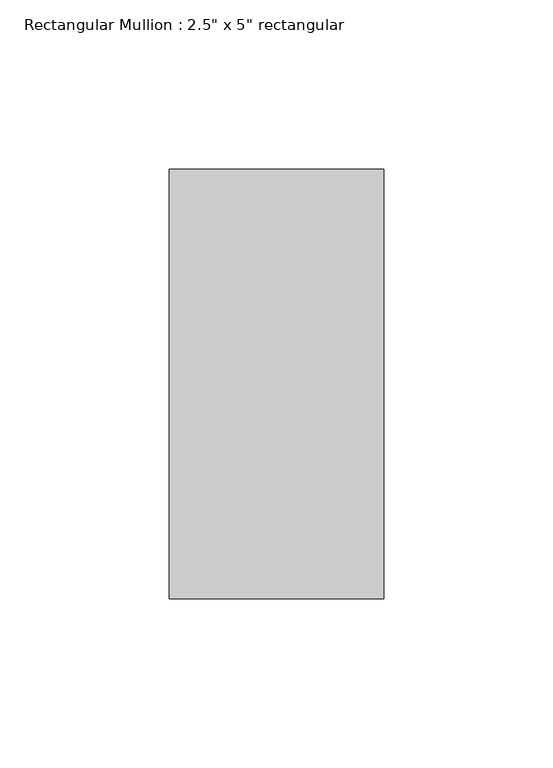
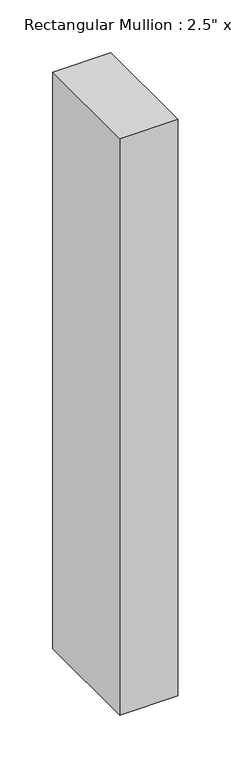
"""IFC4 building model written with IfcOpenShell, lengths in millimetres: member geometry."""

from ifc_helpers import new_model, si_unit, frame, origin, place, context, project, spatial, polyline, outline, extrude, source, transform, mapped, element, save


def member_c33c434a(model_context):
    return source(origin(), model_context, "Body", "SweptSolid", [
        extrude(outline(polyline([(0.0, 63.5), (0.0, -63.5), (-63.5, -63.5), (-63.5, 63.5), (0.0, 63.5)])), frame((0.0, 0.0, -666.75), z_axis=(0.0, 0.0, 1.0), x_axis=(1.0, 0.0, 0.0)), (0.0, 0.0, 1.0), 666.75),
    ])


if __name__ == "__main__":
    model = new_model("IFC4")
    model_context = context("Model", 3, world=origin())
    ifc_project = project(units=[si_unit("LENGTHUNIT", "METRE", prefix="MILLI")], contexts=[model_context])
    site = spatial("IfcSite", under=ifc_project)
    building = spatial("IfcBuilding", under=site)
    placement = place(None, origin())
    member_shape = member_c33c434a(model_context)
    element("IfcMember", 1, ObjectType="Rectangular Mullion : 2.5\" x 5\" rectangular", at=placement, inside=building, context=model_context, shape_type="MappedRepresentation", body=[
        mapped(member_shape, transform((0.0, 0.0, 0.0), x_axis=(1.0, 0.0, 0.0), y_axis=(0.0, 1.0, 0.0), z_axis=(0.0, 0.0, 1.0))),
    ])
    save(model, "model.ifc")

# Revit data of these elements
# Type "Rectangular Mullion : 2.5\" x 5\" rectangular"
#   built-in parameter 1007304 = 0.416667 (stored number, unit not read)
#   built-in parameter 1007301 = 0.104167 (stored number, unit not read)
#   built-in parameter 1007300 = 0.104167 (stored number, unit not read)
# Element 1 (IfcMember, "Rectangular Mullion : 2.5\" x 5\" rectangular")
#   Materials on its faces: "Aluminum"
# Materials
#   "Aluminum": class "Metal", colour RGB 247 247 247, transparency 0, Description = "Aluminum 6061", Cost = 0
